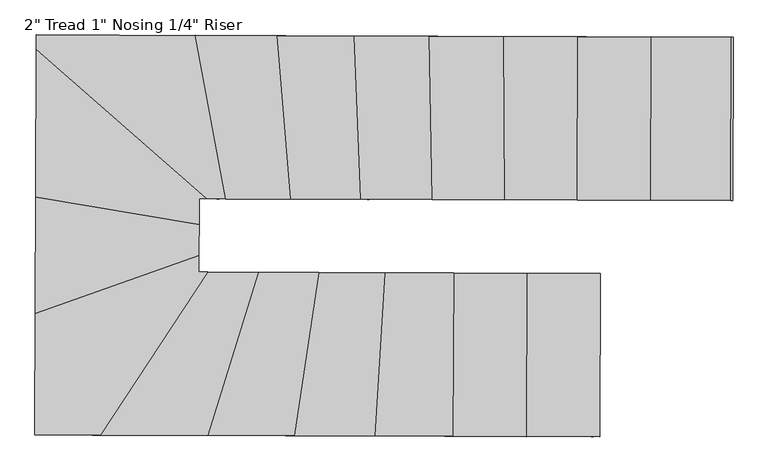
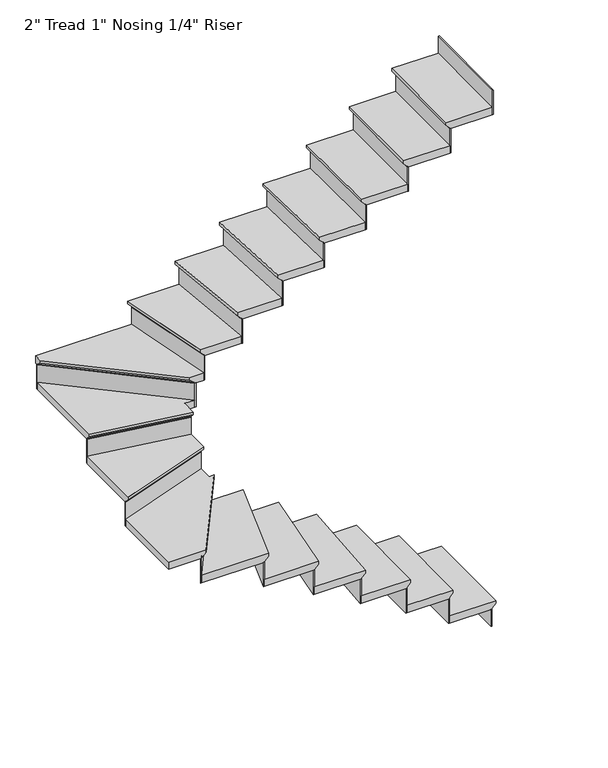
"""IFC4 building model written with IfcOpenShell, lengths in millimetres: stair flight geometry."""

from ifc_helpers import new_model, si_unit, origin, place, context, project, spatial, faceted_brep, source, transform, mapped, element, save


def stair_flight_9e3aa5cb(model_context):
    return source(origin(), model_context, "Body", "Brep", [
        faceted_brep([(-2339.9228929, -4204.0248458, 3350.6833333), (-2339.9228929, -4204.0248458, 3369.7333333), (-2342.0274141, -4826.0015756, 3369.7333333), (-2342.0274141, -4826.0015756, 3350.6833333), (-2365.3227475, -4203.9389029, 3325.2833333), (-2367.4272687, -4825.9156326, 3325.2833333), (-2644.7211481, -4202.9935301, 3369.7333333), (-2646.8256693, -4824.9702599, 3369.7333333), (-2367.4272687, -4825.9156326, 3318.9333333), (-2646.8256693, -4824.9702599, 3318.9333333), (-2644.7211481, -4202.9935301, 3318.9333333), (-2365.3227475, -4203.9389029, 3318.9333333)], [[[0, 1, 2, 3]], [[4, 0, 3, 5]], [[2, 1, 6, 7]], [[8, 9, 10, 11]], [[2, 7, 9, 8, 5, 3]], [[8, 11, 4, 5]], [[6, 1, 0, 4, 11, 10]], [[7, 6, 10, 9]]]),
        faceted_brep([(-2365.3227475, -4203.9389029, 3318.9333333), (-2365.3227475, -4203.9389029, 3200.4), (-2371.6727112, -4203.9174171, 3200.4), (-2371.6727112, -4203.9174171, 3318.9333333), (-2367.4272687, -4825.9156326, 3318.9333333), (-2373.7772323, -4825.8941469, 3318.9333333), (-2373.7772323, -4825.8941469, 3200.4), (-2367.4272687, -4825.9156326, 3200.4)], [[[0, 1, 2, 3]], [[4, 5, 6, 7]], [[1, 0, 4, 7]], [[2, 1, 7, 6]], [[3, 2, 6, 5]], [[0, 3, 5, 4]]]),
        faceted_brep([(-2644.7211481, -4202.9935301, 3488.2666667), (-2644.7211481, -4202.9935301, 3318.9333333), (-2651.0711118, -4202.9720444, 3318.9333333), (-2651.0711118, -4202.9720444, 3488.2666667), (-2646.8256693, -4824.9702599, 3488.2666667), (-2653.175633, -4824.9487741, 3488.2666667), (-2653.175633, -4824.9487741, 3318.9333333), (-2646.8256693, -4824.9702599, 3318.9333333)], [[[0, 1, 2, 3]], [[4, 5, 6, 7]], [[1, 0, 4, 7]], [[2, 1, 7, 6]], [[3, 2, 6, 5]], [[0, 3, 5, 4]]]),
        faceted_brep([(-2621.4258147, -4825.0562028, 3539.0666667), (-2619.3212935, -4203.0794731, 3539.0666667), (-2924.1195488, -4202.0481574, 3539.0666667), (-2926.2240699, -4824.0248871, 3539.0666667), (-2646.8256693, -4824.9702599, 3488.2666667), (-2926.2240699, -4824.0248871, 3488.2666667), (-2924.1195488, -4202.0481574, 3488.2666667), (-2644.7211481, -4202.9935301, 3488.2666667), (-2646.8256693, -4824.9702599, 3494.6166667), (-2621.4258147, -4825.0562028, 3520.0166667), (-2644.7211481, -4202.9935301, 3494.6166667), (-2619.3212935, -4203.0794731, 3520.0166667)], [[[0, 1, 2, 3]], [[4, 5, 6, 7]], [[0, 3, 5, 4, 8, 9]], [[4, 7, 10, 8]], [[2, 1, 11, 10, 7, 6]], [[3, 2, 6, 5]], [[11, 1, 0, 9]], [[10, 11, 9, 8]]]),
        faceted_brep([(-2924.1195488, -4202.0481574, 3657.6), (-2924.1195488, -4202.0481574, 3488.2666667), (-2930.4695124, -4202.0266716, 3488.2666667), (-2930.4695124, -4202.0266716, 3657.6), (-2926.2240699, -4824.0248871, 3657.6), (-2932.5740336, -4824.0034014, 3657.6), (-2932.5740336, -4824.0034014, 3488.2666667), (-2926.2240699, -4824.0248871, 3488.2666667)], [[[0, 1, 2, 3]], [[4, 5, 6, 7]], [[1, 0, 4, 7]], [[2, 1, 7, 6]], [[3, 2, 6, 5]], [[0, 3, 5, 4]]]),
        faceted_brep([(-2900.8242153, -4824.1108301, 3708.4), (-2898.7196941, -4202.1341003, 3708.4), (-3185.4282049, -4201.1639931, 3708.4), (-3223.7984946, -4823.0180139, 3708.4), (-2926.2240699, -4824.0248871, 3657.6), (-3223.7984946, -4823.0180139, 3657.6), (-3185.4282049, -4201.1639931, 3657.6), (-2924.1195488, -4202.0481574, 3657.6), (-2926.2240699, -4824.0248871, 3663.95), (-2900.8242153, -4824.1108301, 3689.35), (-2924.1195488, -4202.0481574, 3663.95), (-2898.7196941, -4202.1341003, 3689.35)], [[[0, 1, 2, 3]], [[4, 5, 6, 7]], [[0, 3, 5, 4, 8, 9]], [[4, 7, 10, 8]], [[2, 1, 11, 10, 7, 6]], [[3, 2, 6, 5]], [[11, 1, 0, 9]], [[10, 11, 9, 8]]]),
        faceted_brep([(-3185.4282049, -4201.1639931, 3826.9333333), (-3185.4282049, -4201.1639931, 3657.6), (-3191.7889535, -4201.1424708, 3657.6), (-3191.7889535, -4201.1424708, 3826.9333333), (-3223.7984946, -4823.0180139, 3826.9333333), (-3230.1592432, -4822.9964917, 3826.9333333), (-3230.1592432, -4822.9964917, 3657.6), (-3223.7984946, -4823.0180139, 3657.6)], [[[0, 1, 2, 3]], [[4, 5, 6, 7]], [[1, 0, 4, 7]], [[2, 1, 7, 6]], [[3, 2, 6, 5]], [[0, 3, 5, 4]]]),
        faceted_brep([(-3198.3555003, -4823.1041029, 3877.7333333), (-3159.9852105, -4201.250082, 3877.7333333), (-3437.1491731, -4200.3122697, 3877.7333333), (-3531.3418182, -4821.97741, 3877.7333333), (-3223.7984946, -4823.0180139, 3826.9333333), (-3531.3418182, -4821.97741, 3826.9333333), (-3437.1491731, -4200.3122697, 3826.9333333), (-3185.4282049, -4201.1639931, 3826.9333333), (-3223.7984946, -4823.0180139, 3833.2833333), (-3198.3555003, -4823.1041029, 3858.6833333), (-3185.4282049, -4201.1639931, 3833.2833333), (-3159.9852105, -4201.250082, 3858.6833333)], [[[0, 1, 2, 3]], [[4, 5, 6, 7]], [[0, 3, 5, 4, 8, 9]], [[4, 7, 10, 8]], [[2, 1, 11, 10, 7, 6]], [[3, 2, 6, 5]], [[11, 1, 0, 9]], [[10, 11, 9, 8]]]),
        faceted_brep([(-3437.1491731, -4200.3122697, 3996.2666667), (-3437.1491731, -4200.3122697, 3826.9333333), (-3443.568358, -4200.2905498, 3826.9333333), (-3443.568358, -4200.2905498, 3996.2666667), (-3531.3418182, -4821.97741, 3996.2666667), (-3537.7610031, -4821.95569, 3996.2666667), (-3537.7610031, -4821.95569, 3826.9333333), (-3531.3418182, -4821.97741, 3826.9333333)], [[[0, 1, 2, 3]], [[4, 5, 6, 7]], [[1, 0, 4, 7]], [[2, 1, 7, 6]], [[3, 2, 6, 5]], [[0, 3, 5, 4]]]),
        faceted_brep([(-3505.6650785, -4822.0642898, 4047.0666667), (-3411.4724335, -4200.3991496, 4047.0666667), (-3668.9000376, -4199.5281172, 4047.0666667), (-3860.1305452, -4820.8649201, 4047.0666667), (-3531.3418182, -4821.97741, 3996.2666667), (-3860.1305452, -4820.8649201, 3996.2666667), (-3668.9000376, -4199.5281172, 3996.2666667), (-3437.1491731, -4200.3122697, 3996.2666667), (-3531.3418182, -4821.97741, 4002.6166667), (-3505.6650785, -4822.0642898, 4028.0166667), (-3437.1491731, -4200.3122697, 4002.6166667), (-3411.4724335, -4200.3991496, 4028.0166667)], [[[0, 1, 2, 3]], [[4, 5, 6, 7]], [[0, 3, 5, 4, 8, 9]], [[4, 7, 10, 8]], [[2, 1, 11, 10, 7, 6]], [[3, 2, 6, 5]], [[11, 1, 0, 9]], [[10, 11, 9, 8]]]),
        faceted_brep([(-3668.9000376, -4199.5281172, 4165.6), (-3668.9000376, -4199.5281172, 3996.2666667), (-3675.5370713, -4199.5056601, 3996.2666667), (-3675.5370713, -4199.5056601, 4165.6), (-3860.1305452, -4820.8649201, 4165.6), (-3866.7675788, -4820.842463, 4165.6), (-3866.7675788, -4820.842463, 3996.2666667), (-3860.1305452, -4820.8649201, 3996.2666667)], [[[0, 1, 2, 3]], [[4, 5, 6, 7]], [[1, 0, 4, 7]], [[2, 1, 7, 6]], [[3, 2, 6, 5]], [[0, 3, 5, 4]]]),
        faceted_brep([(-3833.5824104, -4820.9547484, 4216.4), (-3642.3519028, -4199.6179455, 4216.4), (-3864.4957991, -4198.8662992, 4216.4), (-4274.0422035, -4819.4644081, 4216.4), (-3860.1305452, -4820.8649201, 4165.6), (-4274.0422035, -4819.4644081, 4165.6), (-3864.4957991, -4198.8662992, 4165.6), (-3668.9000376, -4199.5281172, 4165.6), (-3860.1305452, -4820.8649201, 4171.95), (-3833.5824104, -4820.9547484, 4197.35), (-3668.9000376, -4199.5281172, 4171.95), (-3642.3519028, -4199.6179455, 4197.35)], [[[0, 1, 2, 3]], [[4, 5, 6, 7]], [[0, 3, 5, 4, 8, 9]], [[4, 7, 10, 8]], [[2, 1, 11, 10, 7, 6]], [[3, 2, 6, 5]], [[11, 1, 0, 9]], [[10, 11, 9, 8]]]),
        faceted_brep([(-3864.4957991, -4198.8662992, 4334.9333333), (-3864.4957991, -4198.8662992, 4165.6), (-3872.0869257, -4198.8406138, 4165.6), (-3872.0869257, -4198.8406138, 4334.9333333), (-4274.0422035, -4819.4644081, 4334.9333333), (-4281.6333301, -4819.4387227, 4334.9333333), (-4281.6333301, -4819.4387227, 4165.6), (-4274.0422035, -4819.4644081, 4165.6)], [[[0, 1, 2, 3]], [[4, 5, 6, 7]], [[1, 0, 4, 7]], [[2, 1, 7, 6]], [[3, 2, 6, 5]], [[0, 3, 5, 4]]]),
        faceted_brep([(-4490.0684734, -4328.5349965, 4385.7333333), (-4491.7270905, -4818.7278493, 4385.7333333), (-4243.677697, -4819.5671495, 4385.7333333), (-3834.1312926, -4198.9690405, 4385.7333333), (-3867.6458395, -4198.8556407, 4385.7333333), (-3867.338948, -4108.1559559, 4385.7333333), (-4491.7270905, -4818.7278493, 4334.9333333), (-4490.0684734, -4328.5349965, 4334.9333333), (-3867.338948, -4108.1559559, 4334.9333333), (-3867.6458395, -4198.8556407, 4334.9333333), (-3864.4957991, -4198.8662992, 4334.9333333), (-4274.0422035, -4819.4644081, 4334.9333333), (-4274.0422035, -4819.4644081, 4341.2833333), (-4243.677697, -4819.5671495, 4366.6833333), (-3864.4957991, -4198.8662992, 4341.2833333), (-3834.1312926, -4198.9690405, 4366.6833333)], [[[0, 1, 2, 3, 4, 5]], [[6, 7, 8, 9, 10, 11]], [[1, 0, 7, 6]], [[2, 1, 6, 11, 12, 13]], [[11, 10, 14, 12]], [[4, 3, 15, 14, 10, 9]], [[5, 4, 9, 8]], [[0, 5, 8, 7]], [[15, 3, 2, 13]], [[14, 15, 13, 12]]]),
        faceted_brep([(-3867.338948, -4108.1559559, 4504.2666667), (-3867.338948, -4108.1559559, 4334.9333333), (-3867.316129, -4101.4119712, 4334.9333333), (-3867.316129, -4101.4119712, 4504.2666667), (-4490.0684734, -4328.5349965, 4504.2666667), (-4490.0456544, -4321.7910118, 4504.2666667), (-4490.0456544, -4321.7910118, 4334.9333333), (-4490.0684734, -4328.5349965, 4334.9333333)], [[[0, 1, 2, 3]], [[4, 5, 6, 7]], [[1, 0, 4, 7]], [[2, 1, 7, 6]], [[3, 2, 6, 5]], [[0, 3, 5, 4]]]),
        faceted_brep([(-4490.1597492, -4355.5109354, 4555.0666667), (-3867.4302238, -4135.1318948, 4555.0666667), (-3866.9449143, -3991.702012, 4555.0666667), (-4488.5718319, -3886.2129338, 4555.0666667), (-4490.0684734, -4328.5349965, 4504.2666667), (-4488.5718319, -3886.2129338, 4504.2666667), (-3866.9449143, -3991.702012, 4504.2666667), (-3867.338948, -4108.1559559, 4504.2666667), (-4490.0684734, -4328.5349965, 4510.6166667), (-4490.1597492, -4355.5109354, 4536.0166667), (-3867.338948, -4108.1559559, 4510.6166667), (-3867.4302238, -4135.1318948, 4536.0166667)], [[[0, 1, 2, 3]], [[4, 5, 6, 7]], [[0, 3, 5, 4, 8, 9]], [[4, 7, 10, 8]], [[3, 2, 6, 5]], [[11, 1, 0, 9]], [[10, 11, 9, 8]], [[2, 1, 11, 10, 7, 6]]]),
        faceted_brep([(-3866.9449143, -3991.702012, 4673.6), (-3866.9449143, -3991.702012, 4504.2666667), (-3866.9231337, -3985.2649249, 4504.2666667), (-3866.9231337, -3985.2649249, 4673.6), (-4488.5718319, -3886.2129338, 4673.6), (-4488.5500514, -3879.7758467, 4673.6), (-4488.5500514, -3879.7758467, 4504.2666667), (-4488.5718319, -3886.2129338, 4504.2666667)], [[[0, 1, 2, 3]], [[4, 5, 6, 7]], [[1, 0, 4, 7]], [[2, 1, 7, 6]], [[3, 2, 6, 5]], [[0, 3, 5, 4]]]),
        faceted_brep([(-4488.6589541, -3911.9612823, 4724.4), (-3867.0320364, -4017.4503605, 4724.4), (-3866.7004668, -3919.4572401, 4724.4), (-3799.1127501, -3919.6859299, 4724.4), (-4486.6423896, -3315.9795656, 4724.4), (-4488.5718319, -3886.2129338, 4673.6), (-4486.6423896, -3315.9795656, 4673.6), (-3799.1127501, -3919.6859299, 4673.6), (-3866.7004668, -3919.4572401, 4673.6), (-3866.9449143, -3991.702012, 4673.6), (-4488.5718319, -3886.2129338, 4679.95), (-4488.6589541, -3911.9612823, 4705.35), (-3866.9449143, -3991.702012, 4679.95), (-3867.0320364, -4017.4503605, 4705.35)], [[[0, 1, 2, 3, 4]], [[5, 6, 7, 8, 9]], [[0, 4, 6, 5, 10, 11]], [[5, 9, 12, 10]], [[2, 1, 13, 12, 9, 8]], [[4, 3, 7, 6]], [[13, 1, 0, 11]], [[12, 13, 11, 10]], [[3, 2, 8, 7]]]),
        faceted_brep([(-3799.1127501, -3919.6859299, 4842.9333333), (-3799.1127501, -3919.6859299, 4673.6), (-3789.4516067, -3919.7186194, 4673.6), (-3789.4516067, -3919.7186194, 4842.9333333), (-4486.6423896, -3315.9795656, 4842.9333333), (-4486.613881, -3307.5540264, 4842.9333333), (-4486.613881, -3307.5540264, 4673.6), (-4486.6423896, -3315.9795656, 4673.6)], [[[0, 1, 2, 3]], [[4, 5, 6, 7]], [[1, 0, 4, 7]], [[2, 1, 7, 6]], [[3, 2, 6, 5]], [[0, 3, 5, 4]]]),
        faceted_brep([(-3855.3688773, -3297.511731, 4893.7333333), (-4486.5726753, -3295.3759891, 4893.7333333), (-4486.7564243, -3349.6817226, 4893.7333333), (-3837.757324, -3919.5551721, 4893.7333333), (-3739.9081193, -3919.8862548, 4893.7333333), (-4486.5726753, -3295.3759891, 4842.9333333), (-3855.3688773, -3297.511731, 4842.9333333), (-3739.9081193, -3919.8862548, 4842.9333333), (-3799.1127501, -3919.6859299, 4842.9333333), (-4486.6423896, -3315.9795656, 4842.9333333), (-3799.1127501, -3919.6859299, 4849.2833333), (-4486.6423896, -3315.9795656, 4849.2833333), (-3837.757324, -3919.5551721, 4874.6833333), (-4486.7564243, -3349.6817226, 4874.6833333)], [[[0, 1, 2, 3, 4]], [[5, 6, 7, 8, 9]], [[1, 0, 6, 5]], [[9, 8, 10, 11]], [[4, 3, 12, 10, 8, 7]], [[0, 4, 7, 6]], [[12, 3, 2, 13]], [[10, 12, 13, 11]], [[2, 1, 5, 9, 11, 13]]]),
        faceted_brep([(-3739.9081193, -3919.8862548, 5012.2666667), (-3739.9081193, -3919.8862548, 4842.9333333), (-3733.4457151, -3919.908121, 4842.9333333), (-3733.4457151, -3919.908121, 5012.2666667), (-3855.3688773, -3297.511731, 5012.2666667), (-3848.9064731, -3297.5335972, 5012.2666667), (-3848.9064731, -3297.5335972, 4842.9333333), (-3855.3688773, -3297.511731, 4842.9333333)], [[[0, 1, 2, 3]], [[4, 5, 6, 7]], [[1, 0, 4, 7]], [[2, 1, 7, 6]], [[3, 2, 6, 5]], [[0, 3, 5, 4]]]),
        faceted_brep([(-3881.2184941, -3297.4242662, 5063.0666667), (-3765.7577361, -3919.79879, 5063.0666667), (-3493.4024921, -3920.7203315, 5063.0666667), (-3543.7965904, -3298.5659674, 5063.0666667), (-3855.3688773, -3297.511731, 5012.2666667), (-3543.7965904, -3298.5659674, 5012.2666667), (-3493.4024921, -3920.7203315, 5012.2666667), (-3739.9081193, -3919.8862548, 5012.2666667), (-3855.3688773, -3297.511731, 5018.6166667), (-3881.2184941, -3297.4242662, 5044.0166667), (-3739.9081193, -3919.8862548, 5018.6166667), (-3765.7577361, -3919.79879, 5044.0166667)], [[[0, 1, 2, 3]], [[4, 5, 6, 7]], [[0, 3, 5, 4, 8, 9]], [[4, 7, 10, 8]], [[2, 1, 11, 10, 7, 6]], [[3, 2, 6, 5]], [[11, 1, 0, 9]], [[10, 11, 9, 8]]]),
        faceted_brep([(-3493.4024921, -3920.7203315, 5181.6), (-3493.4024921, -3920.7203315, 5012.2666667), (-3487.0299488, -3920.7418937, 5012.2666667), (-3487.0299488, -3920.7418937, 5181.6), (-3543.7965904, -3298.5659674, 5181.6), (-3537.4240471, -3298.5875295, 5181.6), (-3537.4240471, -3298.5875295, 5012.2666667), (-3543.7965904, -3298.5659674, 5012.2666667)], [[[0, 1, 2, 3]], [[4, 5, 6, 7]], [[1, 0, 4, 7]], [[2, 1, 7, 6]], [[3, 2, 6, 5]], [[0, 3, 5, 4]]]),
        faceted_brep([(-3569.2867636, -3298.4797188, 5232.4), (-3518.8926653, -3920.634083, 5232.4), (-3226.664936, -3921.622865, 5232.4), (-3251.8690415, -3299.5537338, 5232.4), (-3543.7965904, -3298.5659674, 5181.6), (-3251.8690415, -3299.5537338, 5181.6), (-3226.664936, -3921.622865, 5181.6), (-3493.4024921, -3920.7203315, 5181.6), (-3543.7965904, -3298.5659674, 5187.95), (-3569.2867636, -3298.4797188, 5213.35), (-3493.4024921, -3920.7203315, 5187.95), (-3518.8926653, -3920.634083, 5213.35)], [[[0, 1, 2, 3]], [[4, 5, 6, 7]], [[0, 3, 5, 4, 8, 9]], [[4, 7, 10, 8]], [[2, 1, 11, 10, 7, 6]], [[3, 2, 6, 5]], [[11, 1, 0, 9]], [[10, 11, 9, 8]]]),
        faceted_brep([(-3226.664936, -3921.622865, 5350.9333333), (-3226.664936, -3921.622865, 5181.6), (-3220.3088547, -3921.6443715, 5181.6), (-3220.3088547, -3921.6443715, 5350.9333333), (-3251.8690415, -3299.5537338, 5350.9333333), (-3245.5129602, -3299.5752402, 5350.9333333), (-3245.5129602, -3299.5752402, 5181.6), (-3251.8690415, -3299.5537338, 5181.6)], [[[0, 1, 2, 3]], [[4, 5, 6, 7]], [[1, 0, 4, 7]], [[2, 1, 7, 6]], [[3, 2, 6, 5]], [[0, 3, 5, 4]]]),
        faceted_brep([(-3277.2933666, -3299.467708, 5401.7333333), (-3252.0892611, -3921.5368393, 5401.7333333), (-2953.9711928, -3922.5455519, 5401.7333333), (-2965.8021755, -3300.52167, 5401.7333333), (-3251.8690415, -3299.5537338, 5350.9333333), (-2965.8021755, -3300.52167, 5350.9333333), (-2953.9711928, -3922.5455519, 5350.9333333), (-3226.664936, -3921.622865, 5350.9333333), (-3251.8690415, -3299.5537338, 5357.2833333), (-3277.2933666, -3299.467708, 5382.6833333), (-3226.664936, -3921.622865, 5357.2833333), (-3252.0892611, -3921.5368393, 5382.6833333)], [[[0, 1, 2, 3]], [[4, 5, 6, 7]], [[0, 3, 5, 4, 8, 9]], [[4, 7, 10, 8]], [[2, 1, 11, 10, 7, 6]], [[3, 2, 6, 5]], [[11, 1, 0, 9]], [[10, 11, 9, 8]]]),
        faceted_brep([(-2953.9711928, -3922.5455519, 5520.2666667), (-2953.9711928, -3922.5455519, 5350.9333333), (-2947.6196355, -3922.567043, 5350.9333333), (-2947.6196355, -3922.567043, 5520.2666667), (-2965.8021755, -3300.52167, 5520.2666667), (-2959.4506182, -3300.5431611, 5520.2666667), (-2959.4506182, -3300.5431611, 5350.9333333), (-2965.8021755, -3300.52167, 5350.9333333)], [[[0, 1, 2, 3]], [[4, 5, 6, 7]], [[1, 0, 4, 7]], [[2, 1, 7, 6]], [[3, 2, 6, 5]], [[0, 3, 5, 4]]]),
        faceted_brep([(-2991.2084046, -3300.4357054, 5571.0666667), (-2979.3774219, -3922.4595874, 5571.0666667), (-2678.7239035, -3923.476879, 5571.0666667), (-2682.2633211, -3301.4810524, 5571.0666667), (-2965.8021755, -3300.52167, 5520.2666667), (-2682.2633211, -3301.4810524, 5520.2666667), (-2678.7239035, -3923.476879, 5520.2666667), (-2953.9711928, -3922.5455519, 5520.2666667), (-2965.8021755, -3300.52167, 5526.6166667), (-2991.2084046, -3300.4357054, 5552.0166667), (-2953.9711928, -3922.5455519, 5526.6166667), (-2979.3774219, -3922.4595874, 5552.0166667)], [[[0, 1, 2, 3]], [[4, 5, 6, 7]], [[0, 3, 5, 4, 8, 9]], [[4, 7, 10, 8]], [[2, 1, 11, 10, 7, 6]], [[3, 2, 6, 5]], [[11, 1, 0, 9]], [[10, 11, 9, 8]]]),
        faceted_brep([(-2678.7239035, -3923.476879, 5689.6), (-2678.7239035, -3923.476879, 5520.2666667), (-2672.3736784, -3923.4983656, 5520.2666667), (-2672.3736784, -3923.4983656, 5689.6), (-2682.2633211, -3301.4810524, 5689.6), (-2675.913096, -3301.502539, 5689.6), (-2675.913096, -3301.502539, 5520.2666667), (-2682.2633211, -3301.4810524, 5520.2666667)], [[[0, 1, 2, 3]], [[4, 5, 6, 7]], [[1, 0, 4, 7]], [[2, 1, 7, 6]], [[3, 2, 6, 5]], [[0, 3, 5, 4]]]),
        faceted_brep([(-2707.6642214, -3301.3951058, 5740.4), (-2704.1248038, -3923.3909324, 5740.4), (-2402.148518, -3924.4126998, 5740.4), (-2400.0439968, -3302.43597, 5740.4), (-2682.2633211, -3301.4810524, 5689.6), (-2400.0439968, -3302.43597, 5689.6), (-2402.148518, -3924.4126998, 5689.6), (-2678.7239035, -3923.476879, 5689.6), (-2682.2633211, -3301.4810524, 5695.95), (-2707.6642214, -3301.3951058, 5721.35), (-2678.7239035, -3923.476879, 5695.95), (-2704.1248038, -3923.3909324, 5721.35)], [[[0, 1, 2, 3]], [[4, 5, 6, 7]], [[0, 3, 5, 4, 8, 9]], [[4, 7, 10, 8]], [[2, 1, 11, 10, 7, 6]], [[3, 2, 6, 5]], [[11, 1, 0, 9]], [[10, 11, 9, 8]]]),
        faceted_brep([(-2402.148518, -3924.4126998, 5858.9333333), (-2402.148518, -3924.4126998, 5689.6), (-2395.7985543, -3924.4341855, 5689.6), (-2395.7985543, -3924.4341855, 5858.9333333), (-2400.0439968, -3302.43597, 5858.9333333), (-2393.6940331, -3302.4574557, 5858.9333333), (-2393.6940331, -3302.4574557, 5689.6), (-2400.0439968, -3302.43597, 5689.6)], [[[0, 1, 2, 3]], [[4, 5, 6, 7]], [[1, 0, 4, 7]], [[2, 1, 7, 6]], [[3, 2, 6, 5]], [[0, 3, 5, 4]]]),
        faceted_brep([(-2425.4438514, -3302.350027, 5909.7333333), (-2427.5483726, -3924.3267568, 5909.7333333), (-2122.7501174, -3925.3580725, 5909.7333333), (-2120.6455962, -3303.3813428, 5909.7333333), (-2400.0439968, -3302.43597, 5858.9333333), (-2120.6455962, -3303.3813428, 5858.9333333), (-2122.7501174, -3925.3580725, 5858.9333333), (-2402.148518, -3924.4126998, 5858.9333333), (-2400.0439968, -3302.43597, 5865.2833333), (-2425.4438514, -3302.350027, 5890.6833333), (-2402.148518, -3924.4126998, 5865.2833333), (-2427.5483726, -3924.3267568, 5890.6833333)], [[[0, 1, 2, 3]], [[4, 5, 6, 7]], [[0, 3, 5, 4, 8, 9]], [[4, 7, 10, 8]], [[2, 1, 11, 10, 7, 6]], [[3, 2, 6, 5]], [[11, 1, 0, 9]], [[10, 11, 9, 8]]]),
        faceted_brep([(-2122.7501174, -3925.3580725, 6028.2666667), (-2122.7501174, -3925.3580725, 5858.9333333), (-2116.4001537, -3925.3795583, 5858.9333333), (-2116.4001537, -3925.3795583, 6028.2666667), (-2120.6455962, -3303.3813428, 6028.2666667), (-2114.2956325, -3303.4028285, 6028.2666667), (-2114.2956325, -3303.4028285, 5858.9333333), (-2120.6455962, -3303.3813428, 5858.9333333)], [[[0, 1, 2, 3]], [[4, 5, 6, 7]], [[1, 0, 4, 7]], [[2, 1, 7, 6]], [[3, 2, 6, 5]], [[0, 3, 5, 4]]]),
        faceted_brep([(-1843.3517167, -3926.3034453, 6197.6), (-1843.3517167, -3926.3034453, 6028.2666667), (-1837.0017531, -3926.324931, 6028.2666667), (-1837.0017531, -3926.324931, 6197.6), (-1841.2471955, -3304.3267155, 6197.6), (-1834.8972319, -3304.3482013, 6197.6), (-1834.8972319, -3304.3482013, 6028.2666667), (-1841.2471955, -3304.3267155, 6028.2666667)], [[[0, 1, 2, 3]], [[4, 5, 6, 7]], [[1, 0, 4, 7]], [[2, 1, 7, 6]], [[3, 2, 6, 5]], [[0, 3, 5, 4]]]),
        faceted_brep([(-2146.0454508, -3303.2953998, 6079.0666667), (-2148.149972, -3925.2721295, 6079.0666667), (-1843.3517167, -3926.3034453, 6079.0666667), (-1841.2471955, -3304.3267155, 6079.0666667), (-2120.6455962, -3303.3813428, 6028.2666667), (-1841.2471955, -3304.3267155, 6028.2666667), (-1843.3517167, -3926.3034453, 6028.2666667), (-2122.7501174, -3925.3580725, 6028.2666667), (-2120.6455962, -3303.3813428, 6034.6166667), (-2146.0454508, -3303.2953998, 6060.0166667), (-2122.7501174, -3925.3580725, 6034.6166667), (-2148.149972, -3925.2721295, 6060.0166667)], [[[0, 1, 2, 3]], [[4, 5, 6, 7]], [[0, 3, 5, 4, 8, 9]], [[4, 7, 10, 8]], [[2, 1, 11, 10, 7, 6]], [[3, 2, 6, 5]], [[11, 1, 0, 9]], [[10, 11, 9, 8]]]),
    ])


if __name__ == "__main__":
    model = new_model("IFC4")
    model_context = context("Model", 3, world=origin())
    ifc_project = project(units=[si_unit("LENGTHUNIT", "METRE", prefix="MILLI")], contexts=[model_context])
    site = spatial("IfcSite", under=ifc_project)
    building = spatial("IfcBuilding", under=site)
    placement = place(None, origin())
    stair_flight_shape = stair_flight_9e3aa5cb(model_context)
    element("IfcStairFlight", 1, ObjectType="2\" Tread 1\" Nosing 1/4\" Riser", at=placement, inside=building, context=model_context, shape_type="MappedRepresentation", body=[
        mapped(stair_flight_shape, transform((0.0, 0.0, 0.0), x_axis=(1.0, 0.0, 0.0), y_axis=(0.0, 1.0, 0.0), z_axis=(0.0, 0.0, 1.0))),
    ])
    save(model, "model.ifc")
